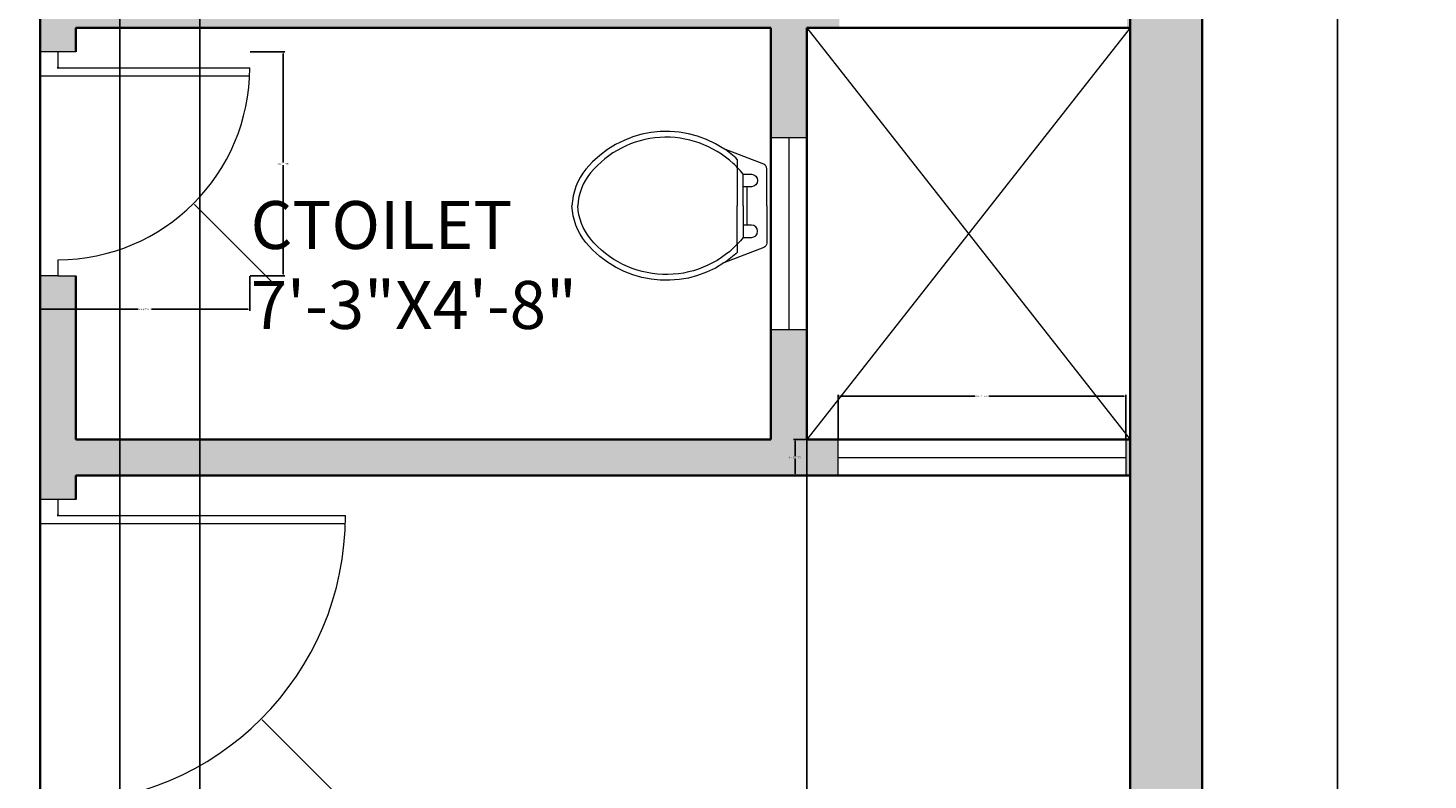
# Model space of a CAD drawing. Units: inches. Extents: x -13 to 349, y -556 to 61.
# Tile 4 of 6: x 170 to 345, y -243 to -149. Entities that reach past the tile are written whole.
import ezdxf

# ---------------------------------------------------------------- set-up
doc = ezdxf.new("R2010")
doc.units = ezdxf.units.IN
doc.header["$MEASUREMENT"] = 0
for name, color, linetype, lineweight in [('A-ANNO-DIMS', 2, 'Continuous', 18), ('A-AREA-IDEN', 7, 'Continuous', 18), ('A-DOOR', 3, 'Continuous', 20), ('A-FLOR-OPEN', 1, 'Continuous', 13), ('A-GLAZ', 5, 'Continuous', 18), ('A-WALL', 7, 'Continuous', 35), ('A-WALL-PATT', 8, 'Continuous', 13), ('WC-Detail_dwgmodels.com', 251, 'Continuous', 13), ('WC-Outline_dwgmodels.com', 250, 'Continuous', 18)]:
    doc.layers.add(name, color=color, linetype=linetype, lineweight=lineweight)
doc.styles.get("Standard").update_dxf_attribs({"font": 'arial.ttf'})
doc.dimstyles.get("Standard").update_dxf_attribs({"dimtxt": 0.18, "dimasz": 0.18, "dimexe": 0.18, "dimexo": 0.0625, "dimgap": 0.09, "dimtad": 0, "dimtih": 1, "dimtoh": 1, "dimdec": 0, "dimzin": 0, "dimdsep": 46, "dimlunit": 3, "dimtxsty": 'Standard', "dimcen": 0.09, "dimadec": 0, "dimazin": 0, "dimtfac": 1, "dimtdec": 0, "dimtofl": 0, "dimtmove": 0, "dimatfit": 3, "dimfxl": 1, "dimtolj": 1, "dimtzin": 0, "dimarcsym": 0})

# ---------------------------------------------------------------- blocks, each defined once
blk = doc.blocks.new('*D3')
at = {"layer": 'A-ANNO-DIMS', "color": 0, "lineweight": -2, "transparency": 16777216}
for p, q in [((316.82, 8.29), (333.9, 8.29)), ((333.72, 8.11), (333.72, -254.62)), ((333.72, -523.53), (333.72, -260.8)), ((316.82, -523.71), (333.9, -523.71))]:
    blk.add_line(p, q, dxfattribs=at)
at = {"layer": 'A-ANNO-DIMS', "color": 0, "transparency": 16777216}
for points in [[(333.69, 8.11), (333.75, 8.11), (333.72, 8.29)], [(333.69, -523.53), (333.75, -523.53), (333.72, -523.71)]]:
    blk.add_solid(points, dxfattribs=at)
at = {"layer": 'Defpoints', "color": 0, "transparency": 16777216}
for p in [(316.76, 8.29), (316.76, -523.71), (333.72, -523.71)]:
    blk.add_point(p, dxfattribs=at)
at = {"layer": 'A-ANNO-DIMS', "color": 0, "transparency": 16777216, "insert": (333.72, -257.71), "char_height": 6, "attachment_point": 5}
blk.add_mtext('\\A1;44\'-4"', dxfattribs=at)
blk = doc.blocks.new('DOOR-SWING-36IN')
for p, q in [((36, 40), (33.75, 40)), ((36, 38), (36, 40)), ((36, 40), (38.25, 40)), ((38.25, 3), (0, 3)), ((36, 2), (0, 2)), ((36, 0), (36, 2)), ((33.75, 0), (38.25, 0))]:
    blk.add_line(p, q)
blk.add_arc((36, 2), 36, 90, 180)
blk = doc.blocks.new('DOOR-SWING-24IN')
for p, q in [((4.5, 28), (0, 28)), ((2.25, 28), (2.25, 26)), ((0, 25), (26.25, 25)), ((2.25, 26), (26.25, 26)), ((2.25, 2), (2.25, 0)), ((2.25, 0), (0, 0)), ((2.25, 0), (4.5, 0))]:
    blk.add_line(p, q)
blk.add_arc((2.25, 26), 24, 270, 0)
blk = doc.blocks.new('WIN-36IN-D4_5')
for p, q in [((0, 4.5), (36, 4.5)), ((0, 0), (0, 4.5)), ((36, 4.5), (36, 0)), ((0, 2.25), (36, 2.25)), ((36, 0), (0, 0))]:
    blk.add_line(p, q)
blk = doc.blocks.new('*D16')
at = {"layer": 'A-ANNO-DIMS', "color": 0, "lineweight": -2, "transparency": 16777216}
for p, q in [((197.57, -152.21), (201.89, -152.21)), ((201.71, -152.39), (201.71, -166.03)), ((201.71, -180.03), (201.71, -166.39)), ((197.57, -180.21), (201.89, -180.21))]:
    blk.add_line(p, q, dxfattribs=at)
at = {"layer": 'A-ANNO-DIMS', "color": 0, "transparency": 16777216}
for points in [[(201.68, -152.39), (201.74, -152.39), (201.71, -152.21)], [(201.68, -180.03), (201.74, -180.03), (201.71, -180.21)]]:
    blk.add_solid(points, dxfattribs=at)
at = {"layer": 'Defpoints', "color": 0, "transparency": 16777216}
for p in [(197.51, -152.21), (201.71, -152.21), (197.51, -180.21)]:
    blk.add_point(p, dxfattribs=at)
at = {"layer": 'A-ANNO-DIMS', "color": 0, "transparency": 16777216, "insert": (201.71, -166.21), "char_height": 0.18, "attachment_point": 5}
blk.add_mtext('\\A1;D2 2\'-4" TYP.', dxfattribs=at)
blk = doc.blocks.new('*D17')
at = {"layer": 'A-ANNO-DIMS', "color": 0, "lineweight": -2, "transparency": 16777216}
for p, q in [((171.26, -180.28), (171.26, -184.59)), ((197.51, -180.28), (197.51, -184.59)), ((171.44, -184.41), (183.53, -184.41)), ((197.33, -184.41), (185.23, -184.41))]:
    blk.add_line(p, q, dxfattribs=at)
at = {"layer": 'A-ANNO-DIMS', "color": 0, "transparency": 16777216}
for points in [[(171.44, -184.38), (171.44, -184.44), (171.26, -184.41)], [(197.33, -184.38), (197.33, -184.44), (197.51, -184.41)]]:
    blk.add_solid(points, dxfattribs=at)
at = {"layer": 'Defpoints', "color": 0, "transparency": 16777216}
for p in [(171.26, -180.21), (197.51, -180.21), (197.51, -184.41)]:
    blk.add_point(p, dxfattribs=at)
at = {"layer": 'A-ANNO-DIMS', "color": 0, "transparency": 16777216, "insert": (184.38, -184.41), "char_height": 0.18, "attachment_point": 5}
blk.add_mtext('\\A1;2\'-2 1/2" TYP.', dxfattribs=at)
blk = doc.blocks.new('*D24')
at = {"layer": 'A-ANNO-DIMS', "color": 0, "lineweight": -2, "transparency": 16777216}
for p, q in [((271.19, -200.65), (271.19, -195.13)), ((271.37, -195.31), (288.33, -195.31)), ((307.01, -195.31), (290.06, -195.31)), ((307.19, -200.65), (307.19, -195.13))]:
    blk.add_line(p, q, dxfattribs=at)
at = {"layer": 'A-ANNO-DIMS', "color": 0, "transparency": 16777216}
for points in [[(271.37, -195.28), (271.37, -195.34), (271.19, -195.31)], [(307.01, -195.28), (307.01, -195.34), (307.19, -195.31)]]:
    blk.add_solid(points, dxfattribs=at)
at = {"layer": 'Defpoints', "color": 0, "transparency": 16777216}
for p in [(307.19, -195.31), (271.19, -200.71), (307.19, -200.71)]:
    blk.add_point(p, dxfattribs=at)
at = {"layer": 'A-ANNO-DIMS', "color": 0, "transparency": 16777216, "insert": (289.19, -195.31), "char_height": 0.18, "attachment_point": 5}
blk.add_mtext('\\A1;W4 3\'-0" TYP.', dxfattribs=at)
blk = doc.blocks.new('*D25')
at = {"layer": 'A-ANNO-DIMS', "color": 0, "lineweight": -2, "transparency": 16777216}
for p, q in [((271.13, -200.71), (265.61, -200.71)), ((265.79, -200.89), (265.79, -202.78)), ((265.79, -205.03), (265.79, -203.15)), ((271.13, -205.21), (265.61, -205.21))]:
    blk.add_line(p, q, dxfattribs=at)
at = {"layer": 'A-ANNO-DIMS', "color": 0, "transparency": 16777216}
for points in [[(265.76, -200.89), (265.82, -200.89), (265.79, -200.71)], [(265.76, -205.03), (265.82, -205.03), (265.79, -205.21)]]:
    blk.add_solid(points, dxfattribs=at)
at = {"layer": 'Defpoints', "color": 0, "transparency": 16777216}
for p in [(265.79, -200.71), (271.19, -200.71), (271.19, -205.21)]:
    blk.add_point(p, dxfattribs=at)
at = {"layer": 'A-ANNO-DIMS', "color": 0, "transparency": 16777216, "insert": (265.79, -202.96), "char_height": 0.18, "attachment_point": 5}
blk.add_mtext('\\A1;0\'-4 1/2" TYP.', dxfattribs=at)
blk = doc.blocks.new('*D34')
at = {"layer": 'A-ANNO-DIMS', "color": 0, "lineweight": -2, "transparency": 16777216}
for p, q in [((267.26, -200.78), (267.26, -555.89)), ((307.76, -200.78), (307.76, -555.89)), ((267.44, -555.71), (286.97, -555.71)), ((307.58, -555.71), (288.04, -555.71))]:
    blk.add_line(p, q, dxfattribs=at)
at = {"layer": 'A-ANNO-DIMS', "color": 0, "transparency": 16777216}
for points in [[(267.44, -555.68), (267.44, -555.74), (267.26, -555.71)], [(307.58, -555.68), (307.58, -555.74), (307.76, -555.71)]]:
    blk.add_solid(points, dxfattribs=at)
at = {"layer": 'Defpoints', "color": 0, "transparency": 16777216}
for p in [(267.26, -200.71), (307.76, -200.71), (307.76, -555.71)]:
    blk.add_point(p, dxfattribs=at)
at = {"layer": 'A-ANNO-DIMS', "color": 0, "transparency": 16777216, "insert": (287.51, -555.71), "char_height": 0.18, "attachment_point": 5}
blk.add_mtext('\\A1;3\'-4 1/2"', dxfattribs=at)
blk = doc.blocks.new('*D37')
at = {"layer": 'A-ANNO-DIMS', "color": 0, "lineweight": -2, "transparency": 16777216}
for p, q in [((181.26, -353.65), (181.26, 40.47)), ((191.26, -353.65), (191.26, 40.47)), ((181.44, 40.29), (185.86, 40.29)), ((191.08, 40.29), (186.65, 40.29))]:
    blk.add_line(p, q, dxfattribs=at)
at = {"layer": 'A-ANNO-DIMS', "color": 0, "transparency": 16777216}
for points in [[(181.44, 40.32), (181.44, 40.26), (181.26, 40.29)], [(191.08, 40.32), (191.08, 40.26), (191.26, 40.29)]]:
    blk.add_solid(points, dxfattribs=at)
at = {"layer": 'Defpoints', "color": 0, "transparency": 16777216}
for p in [(191.26, 40.29), (181.26, -353.71), (191.26, -353.71)]:
    blk.add_point(p, dxfattribs=at)
at = {"layer": 'A-ANNO-DIMS', "color": 0, "transparency": 16777216, "insert": (186.26, 40.29), "char_height": 0.18, "attachment_point": 5}
blk.add_mtext('\\A1;0\'-10"', dxfattribs=at)
blk = doc.blocks.new('*D48')
at = {"layer": 'A-ANNO-DIMS', "color": 0, "lineweight": -2, "transparency": 16777216}
for p, q in [((173.42, -210.21), (173.6, -210.21)), ((173.51, -210.3), (173.51, -210.12)), ((214.24, -250.94), (199.09, -235.8)), ((214.42, -250.94), (214.24, -250.94))]:
    blk.add_line(p, q, dxfattribs=at)
at = {"layer": 'A-ANNO-DIMS', "color": 0, "transparency": 16777216}
blk.add_solid([(199.11, -235.77), (199.07, -235.82), (198.96, -235.67)], dxfattribs=at)
at = {"layer": 'Defpoints', "color": 0, "transparency": 16777216}
for p in [(173.51, -210.21), (198.96, -235.67)]:
    blk.add_point(p, dxfattribs=at)
at = {"layer": 'A-ANNO-DIMS', "color": 0, "transparency": 16777216, "insert": (215.03, -250.94), "char_height": 0.18, "attachment_point": 5}
blk.add_mtext('\\A1;4X R3\'-0"', dxfattribs=at)
blk = doc.blocks.new('*D49')
at = {"layer": 'A-ANNO-DIMS', "color": 0, "lineweight": -2, "transparency": 16777216}
for p, q in [((173.42, -154.21), (173.6, -154.21)), ((173.51, -154.3), (173.51, -154.12)), ((200.66, -181.37), (190.6, -171.31)), ((200.84, -181.37), (200.66, -181.37))]:
    blk.add_line(p, q, dxfattribs=at)
at = {"layer": 'A-ANNO-DIMS', "color": 0, "transparency": 16777216}
blk.add_solid([(190.62, -171.29), (190.58, -171.33), (190.48, -171.18)], dxfattribs=at)
at = {"layer": 'Defpoints', "color": 0, "transparency": 16777216}
for p in [(173.51, -154.21), (190.48, -171.18)]:
    blk.add_point(p, dxfattribs=at)
at = {"layer": 'A-ANNO-DIMS', "color": 0, "transparency": 16777216, "insert": (201.45, -181.37), "char_height": 0.18, "attachment_point": 5}
blk.add_mtext('\\A1;3X R2\'-0"', dxfattribs=at)

msp = doc.modelspace()

# ---------------------------------------------------------------- hatches: boundary and pattern name
at = {"layer": 'A-WALL-PATT'}
h = msp.add_hatch(color=256, dxfattribs=at)
h.dxf.hatch_style = 1
h.paths.add_polyline_path([(316.76, 8.29), (171.26, 8.29), (171.26, -0.71), (307.76, -0.71), (307.76, -52.19), (316.76, -52.19)])
h.paths.add_polyline_path([(175.76, -0.71), (171.26, -0.71), (171.26, -82.21), (165.24, -82.21), (165.24, -86.71), (171.26, -86.71), (171.26, -101.71), (173.51, -101.71), (175.76, -101.71)])
h.paths.add_polyline_path([(171.26, -25.21), (165.17, -25.21), (165.17, -34.21), (171.26, -34.21)])
h.paths.add_polyline_path([(141.17, -25.21), (127.76, -25.21), (127.76, -34.21), (141.17, -34.21)])
h.paths.add_polyline_path([(28.76, -25.21), (24.26, -25.21), (19.76, -25.21), (19.76, -78.88), (28.76, -78.88)])
h.paths.add_polyline_path([(99.76, -29.71), (99.76, -25.21), (28.76, -25.21), (28.76, -34.21), (99.76, -34.21)])
h.paths.add_polyline_path([(135.26, -86.71), (143.68, -86.71), (143.68, -82.21), (135.26, -82.21), (135.26, -34.21), (130.76, -34.21), (130.76, -101.71), (133.01, -101.71), (135.26, -101.71)])
h.paths.add_polyline_path([(135.26, -141.71), (130.76, -141.71), (130.76, -144.71), (28.76, -144.71), (28.76, -149.21), (135.26, -149.21)])
h.paths.add_polyline_path([(28.76, -138.88), (19.76, -138.88), (19.76, -156.62), (28.76, -156.62)])
h.paths.add_polyline_path([(28.76, -192.62), (19.76, -192.62), (19.76, -271.06), (28.76, -271.06)])
h.paths.add_polyline_path([(28.76, -307.06), (19.76, -307.06), (19.76, -385.56), (28.76, -385.56)])
h.paths.add_polyline_path([(28.76, -445.56), (19.76, -445.56), (19.76, -523.71), (28.76, -523.71)])
h.paths.add_polyline_path([(307.76, -431.71), (261.76, -431.71), (261.76, -353.71), (264.76, -353.71), (264.76, -349.21), (175.76, -349.21), (175.76, -248.21), (173.51, -248.21), (171.26, -248.21), (171.26, -317.21), (168.26, -317.21), (168.26, -321.71), (171.26, -321.71), (171.26, -353.71), (257.26, -353.71), (257.26, -431.71), (171.26, -431.71), (171.26, -436.21), (307.76, -436.21)])
h.paths.add_polyline_path([(316.76, -424.85), (307.76, -424.85), (307.76, -436.21), (316.76, -436.21)])
h.paths.add_polyline_path([(316.76, -305.84), (307.76, -305.84), (307.76, -400.85), (316.76, -400.85)])
h.paths.add_polyline_path([(307.76, -349.21), (292.76, -349.21), (292.76, -351.46), (292.76, -353.71), (307.76, -353.71)], flags=17)
h.paths.add_polyline_path([(271.19, -200.71), (267.26, -200.71), (267.26, -186.96), (262.76, -186.96), (262.76, -200.71), (175.76, -200.71), (175.76, -180.21), (173.51, -180.21), (171.26, -180.21), (171.26, -208.21), (175.76, -208.21), (175.76, -205.21), (271.19, -205.21)])
h.paths.add_polyline_path([(316.76, -112.19), (307.76, -112.19), (307.76, -245.84), (316.76, -245.84)])
h.paths.add_polyline_path([(271.33, -144.71), (175.76, -144.71), (175.76, -141.71), (171.26, -141.71), (171.26, -152.21), (175.76, -152.21), (175.76, -149.21), (262.76, -149.21), (262.76, -162.96), (267.26, -162.96), (267.26, -149.21), (271.33, -149.21)])
h.paths.add_polyline_path([(307.76, -200.71), (307.19, -200.71), (307.19, -205.21), (307.76, -205.21)])
h.paths.add_polyline_path([(307.76, -144.71), (307.33, -144.71), (307.33, -149.21), (307.76, -149.21)])

# ---------------------------------------------------------------- linework, layer by layer
at = {"layer": 'A-FLOR-OPEN'}
for p, q in [((267.26, -149.21), (307.76, -200.71)), ((307.76, -149.21), (267.26, -200.71))]:
    msp.add_line(p, q, dxfattribs=at)
at = {"layer": 'A-GLAZ'}
for p, q in [((262.76, -162.96), (262.76, -186.96)), ((267.26, -162.96), (262.76, -162.96)), ((265.01, -162.96), (265.01, -186.96)), ((267.26, -186.96), (267.26, -162.96)), ((262.76, -186.96), (267.26, -186.96))]:
    msp.add_line(p, q, dxfattribs=at)
at = {"layer": 'A-WALL'}
for p, q in [((316.76, 8.29), (316.76, -523.71)), ((307.76, -0.71), (307.76, -436.21)), ((171.26, -86.71), (171.26, -317.21)), ((175.76, -149.21), (175.76, -152.21)), ((175.76, -149.21), (262.76, -149.21)), ((262.76, -149.21), (262.76, -200.71)), ((267.26, -149.21), (267.26, -200.71)), ((267.26, -149.21), (307.76, -149.21)), ((175.76, -180.21), (175.76, -200.71)), ((175.76, -200.71), (262.76, -200.71)), ((267.26, -200.71), (307.76, -200.71)), ((175.76, -205.21), (175.76, -208.21)), ((175.76, -205.21), (307.76, -205.21))]:
    msp.add_line(p, q, dxfattribs=at)
at = {"layer": 'WC-Detail_dwgmodels.com'}
for p, q in [((258.56, -165.65), (258.56, -166.67)), ((258.56, -176.27), (258.56, -177.3))]:
    msp.add_line(p, q, dxfattribs=at)
for points in [[(258.56, -165.65, 0.040937), (256.88, -164.33, 0.163732)], [(259.3, -167.52, 0.022712), (258.56, -166.67, 0.162618)], [(259.3, -171.47), (259.3, -167.52, 0.022712)], [(259.3, -167.52), (260.32, -167.52, -1), (260.32, -169.07), (259.79, -169.07)], [(259.3, -171.47), (259.3, -175.43, -0.476108)], [(259.3, -175.43), (260.32, -175.43, 1), (260.32, -173.88), (259.79, -173.88)], [(259.3, -175.43, -0.022712), (258.56, -176.27, -0.162618)], [(258.56, -177.3, -0.040937), (256.88, -178.62, -0.163732)]]:
    msp.add_lwpolyline(points, format="xyb", dxfattribs=at)
for points in [[(259.79, -169.07), (259.3, -169.07)], [(259.79, -173.88), (259.79, -169.07)], [(259.79, -173.88), (259.3, -173.88)]]:
    msp.add_lwpolyline(points, dxfattribs=at)
at = {"layer": 'WC-Outline_dwgmodels.com'}
for p in [(258.56, -166.67), (258.56, -176.27)]:
    msp.add_line(p, (258.56, -171.47), dxfattribs=at)
for points in [[(256.88, -164.33, 0.383919), (239.61, -166.89, 0.163732), (237.86, -171.47, 0.359733)], [(258.06, -166.19, 0.431639), (240.18, -167.35, 0.162618), (238.59, -171.47, 0.470877)], [(262.25, -171.47), (262.25, -166.82, 0.31031), (261.86, -166.24), (256.88, -164.33, 0.209071)], [(258.56, -166.67, 0.014165), (258.06, -166.19, 0.162618)], [(256.88, -178.62, -0.383919), (239.61, -176.06, -0.163732), (237.86, -171.47, -0.359733)], [(258.56, -176.27, -0.448546), (240.18, -175.6, -0.162618), (238.59, -171.47, -0.470877)], [(262.25, -171.47), (262.25, -176.13, -0.31031), (261.86, -176.7), (256.88, -178.62, -0.209071)]]:
    msp.add_lwpolyline(points, format="xyb", dxfattribs=at)

# ---------------------------------------------------------------- block references
at = {"layer": 'A-DOOR'}
msp.add_blockref('DOOR-SWING-24IN', (171.26, -180.21), dxfattribs=at)
at = {"layer": 'A-DOOR', "rotation": 180}
msp.add_blockref('DOOR-SWING-36IN', (209.5, -208.22), dxfattribs=at)
at = {"layer": 'A-GLAZ'}
msp.add_blockref('WIN-36IN-D4_5', (271.19, -205.21), dxfattribs=at)

# ---------------------------------------------------------------- texts
at = {"layer": 'A-AREA-IDEN', "insert": (197.63, -170.87), "char_height": 6, "attachment_point": 1}
msp.add_mtext_dynamic_manual_height_columns('CTOILET\\P7\'-3"X4\'-8"', width=1.4038, gutter_width=1, heights=[0], dxfattribs=at)

# ---------------------------------------------------------------- dimensions: what is measured, and where the dimension line sits
at = {"layer": 'A-ANNO-DIMS'}
for base, p1, p2, picture, middle in [((191.26, 40.29), (181.26, -353.71), (191.26, -353.71), '*D37', (186.26, 40.29)), ((307.76, -555.71), (267.26, -200.71), (307.76, -200.71), '*D34', (287.51, -555.71))]:
    dim = msp.add_linear_dim(base=base, p1=p1, p2=p2, dimstyle='Standard', override={"dimdec": 1, "dimlfac": 1, "dimrnd": 0, "dimzin": 1, "dimdsep": 46, "dimlunit": 4, "dimfrac": 2}, dxfattribs=at)
    dim.commit()
    dim.dimension.update_dxf_attribs({"geometry": picture, "text_midpoint": middle})
dim = msp.add_linear_dim(base=(333.72, -523.71), p1=(316.76, 8.29), p2=(316.76, -523.71), angle=90, dimstyle='Standard', override={"dimtxt": 6, "dimclrd": 0, "dimclre": 0, "dimclrt": 0}, dxfattribs=at)
dim.commit()
dim.dimension.update_dxf_attribs({"geometry": '*D3', "text_midpoint": (333.72, -257.71)})
for base, p1, p2, text, picture, middle in [((201.71, -152.21), (197.51, -180.21), (197.51, -152.21), 'D2 <> TYP.', '*D16', (201.71, -166.21)), ((265.79, -200.71), (271.19, -205.21), (271.19, -200.71), '<> TYP.', '*D25', (265.79, -202.96))]:
    dim = msp.add_linear_dim(base=base, p1=p1, p2=p2, angle=90, text=text, dimstyle='Standard', override={"dimdec": 1, "dimlfac": 1, "dimrnd": 0, "dimzin": 1, "dimdsep": 46, "dimlunit": 4, "dimfrac": 2}, dxfattribs=at)
    dim.commit()
    dim.dimension.update_dxf_attribs({"geometry": picture, "text_midpoint": middle})
for center, mpoint, text, picture, middle in [((173.51, -154.21), (190.48, -171.18), '3X <>', '*D49', (201.45, -181.37)), ((173.51, -210.21), (198.96, -235.67), '4X <>', '*D48', (215.03, -250.94))]:
    dim = msp.add_radius_dim(center=center, mpoint=mpoint, text=text, dimstyle='Standard', override={"dimdec": 1, "dimlfac": 1, "dimrnd": 0, "dimzin": 1, "dimdsep": 46, "dimlunit": 4, "dimfrac": 2}, dxfattribs=at)
    dim.commit()
    dim.dimension.update_dxf_attribs({"geometry": picture, "text_midpoint": middle, "dimtype": 164})
for base, p1, p2, text, picture, middle in [((197.50577516, -184.41326771), (171.25577516, -180.21326771), (197.50577516, -180.21326771), '<> TYP.', '*D17', (184.38077516, -184.41326771)), ((307.19, -195.31), (271.19, -200.71), (307.19, -200.71), 'W4 <> TYP.', '*D24', (289.19, -195.31))]:
    dim = msp.add_linear_dim(base=base, p1=p1, p2=p2, text=text, dimstyle='Standard', override={"dimdec": 1, "dimlfac": 1, "dimrnd": 0, "dimzin": 1, "dimdsep": 46, "dimlunit": 4, "dimfrac": 2}, dxfattribs=at)
    dim.commit()
    dim.dimension.update_dxf_attribs({"geometry": picture, "text_midpoint": middle})

doc.saveas('drawing.dxf')
